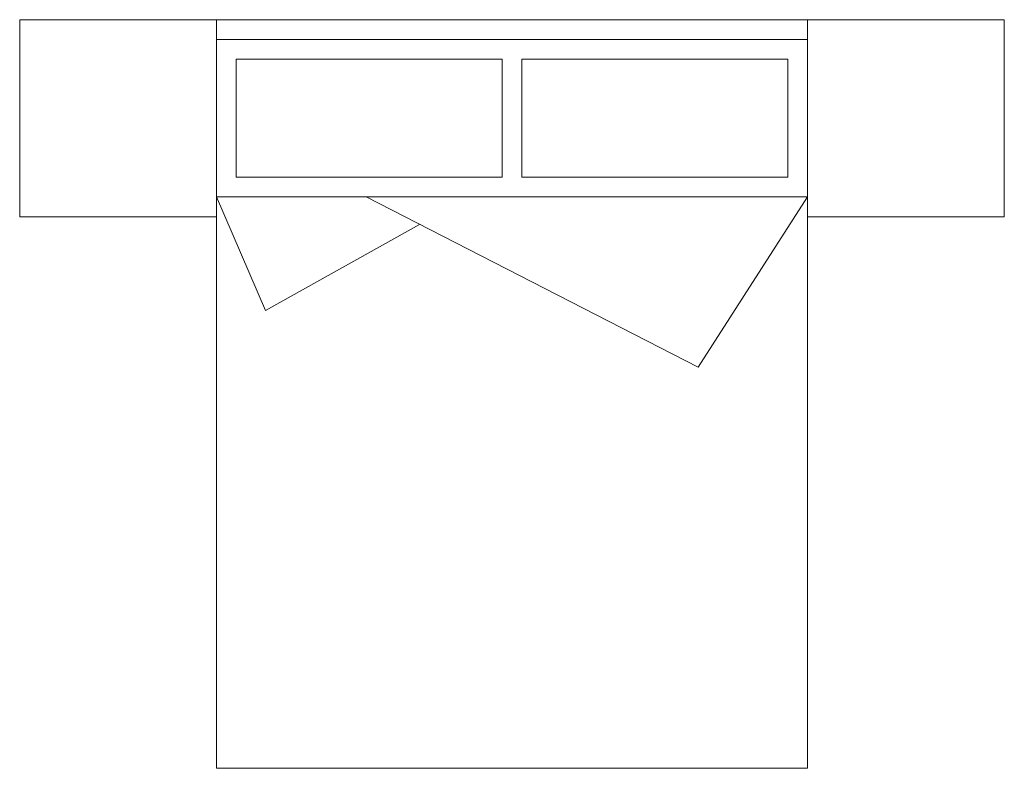
# Model space of a CAD drawing. Units: inches. Extents: x 1994 to 3075, y 3517 to 3950.
# Tile 22 of 58: x 1994.24162 to 1994.34005, y 3553.6999 to 3553.7747. Entities that reach past the tile are written whole.
import ezdxf

# ---------------------------------------------------------------- set-up
doc = ezdxf.new("R2010")
doc.units = ezdxf.units.IN
doc.layers.add('A-FURN-REFR', color=8, linetype='Continuous', lineweight=13)

msp = doc.modelspace()

# ---------------------------------------------------------------- linework, layer by layer
at = {"layer": 'A-FURN-REFR'}
for p, q in [((1994.320364, 3553.774705), (1994.261309, 3553.774705)), ((1994.261309, 3553.774705), (1994.261309, 3553.699901)), ((1994.320364, 3553.774705), (1994.320364, 3553.699901)), ((1994.320364, 3553.772736), (1994.261309, 3553.772736)), ((1994.289853, 3553.770768), (1994.263278, 3553.770768)), ((1994.263278, 3553.770768), (1994.263278, 3553.758956)), ((1994.289853, 3553.770768), (1994.289853, 3553.758956)), ((1994.291821, 3553.770768), (1994.291821, 3553.758956)), ((1994.318396, 3553.770768), (1994.291821, 3553.770768)), ((1994.318396, 3553.770768), (1994.318396, 3553.758956)), ((1994.289853, 3553.758956), (1994.263278, 3553.758956)), ((1994.318396, 3553.758956), (1994.291821, 3553.758956)), ((1994.320364, 3553.756988), (1994.261309, 3553.756988)), ((1994.266212, 3553.745634), (1994.261309, 3553.756988)), ((1994.309453, 3553.739968), (1994.276245, 3553.756988)), ((1994.320364, 3553.756988), (1994.309453, 3553.739968)), ((1994.281599, 3553.754244), (1994.266212, 3553.745634)), ((1994.320364, 3553.699901), (1994.261309, 3553.699901))]:
    msp.add_line(p, q, dxfattribs=at)
for points in [[(1994.241624, 3553.755019), (1994.261309, 3553.755019), (1994.261309, 3553.774705), (1994.241624, 3553.774705)], [(1994.340049, 3553.755019), (1994.320364, 3553.755019), (1994.320364, 3553.774705), (1994.340049, 3553.774705)]]:
    msp.add_lwpolyline(points, close=True, dxfattribs=at)

doc.saveas('drawing.dxf')
